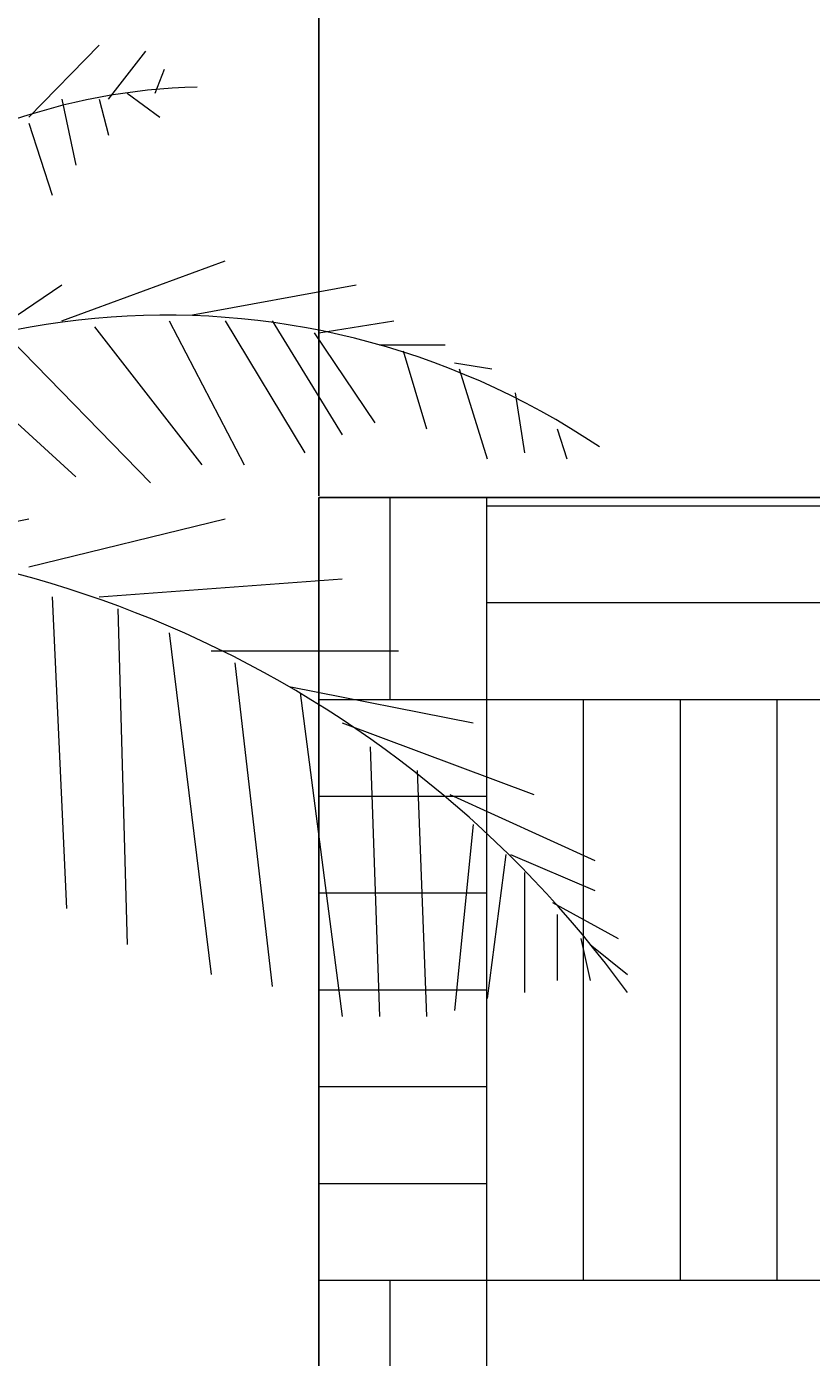
# Model space of a CAD drawing. Units: inches. Extents: x 37 to 824, y -700 to 234.
# Tile 6 of 77: x 149 to 181, y -459 to -404. Entities that reach past the tile are written whole.
import ezdxf

# ---------------------------------------------------------------- set-up
doc = ezdxf.new("R2010")
doc.units = ezdxf.units.IN
doc.header["$MEASUREMENT"] = 0
for name, color, linetype, lineweight in [('A-ANNO-DIMS', 2, 'Continuous', 18), ('A-ELEV', 3, 'Continuous', 25), ('A-ELEV-PATT', 8, 'Continuous', 13), ('A-SITE-PLNT', 3, 'Continuous', 13)]:
    doc.layers.add(name, color=color, linetype=linetype, lineweight=lineweight)
doc.styles.get("Standard").update_dxf_attribs({"font": 'arial.ttf'})
doc.dimstyles.get("Standard").update_dxf_attribs({"dimtxt": 0.18, "dimasz": 0.18, "dimexe": 0.18, "dimexo": 0.0625, "dimgap": 0.09, "dimtad": 0, "dimtih": 1, "dimtoh": 1, "dimdec": 1, "dimzin": 0, "dimdsep": 46, "dimlunit": 4, "dimtxsty": 'Standard', "dimcen": 0.09, "dimadec": 0, "dimazin": 0, "dimtfac": 1, "dimtdec": 1, "dimtofl": 0, "dimtmove": 0, "dimatfit": 3, "dimfxl": 1, "dimtolj": 1, "dimtzin": 0, "dimarcsym": 0})

# ---------------------------------------------------------------- blocks, each defined once
blk = doc.blocks.new('*U34')
for p, q in [((18.015, 195.716), (20.914, 198.689)), ((21.301, 196.459), (22.847, 198.441)), ((23.234, 196.707), (23.62, 197.698)), ((19.368, 196.459), (19.948, 193.733)), ((20.914, 196.459), (21.301, 194.972)), ((22.074, 196.707), (23.427, 195.716)), ((18.015, 195.468), (18.981, 192.494)), ((19.368, 187.29), (26.133, 189.768)), ((15.695, 186.299), (19.368, 188.777)), ((24.78, 187.538), (31.546, 188.777)), ((20.721, 187.042), (25.167, 181.343)), ((23.814, 187.29), (26.907, 181.343)), ((26.133, 187.29), (29.419, 181.838)), ((28.066, 187.29), (30.966, 182.582)), ((29.999, 186.795), (33.092, 187.29)), ((17.242, 186.547), (23.041, 180.599)), ((29.806, 186.795), (32.319, 183.078)), ((32.512, 186.299), (35.218, 186.299)), ((33.479, 186.051), (34.445, 182.83)), ((14.536, 185.803), (19.948, 180.847)), ((35.605, 185.556), (37.151, 185.308)), ((35.798, 185.308), (36.958, 181.591)), ((38.118, 184.317), (38.504, 181.838)), ((39.857, 182.83), (40.244, 181.591)), ((11.829, 177.874), (18.015, 179.113)), ((18.015, 177.13), (26.133, 179.113)), ((20.914, 175.891), (30.966, 176.635)), ((18.981, 175.891), (19.561, 163.005)), ((21.688, 175.396), (22.074, 161.518)), ((23.814, 174.404), (25.554, 160.279)), ((25.554, 173.661), (33.285, 173.661)), ((26.52, 173.165), (28.066, 159.784)), ((28.839, 172.174), (36.378, 170.687)), ((29.226, 171.926), (30.966, 158.545)), ((30.966, 170.687), (38.891, 167.713)), ((32.126, 169.696), (32.512, 158.545)), ((34.058, 168.705), (34.445, 158.545)), ((35.412, 167.713), (41.404, 164.988)), ((36.378, 166.474), (35.605, 158.792)), ((37.731, 165.235), (36.958, 159.288)), ((37.924, 165.235), (41.404, 163.749)), ((38.504, 164.492), (38.504, 159.536)), ((39.664, 163.253), (42.37, 161.766)), ((39.857, 162.757), (39.857, 160.031)), ((40.824, 161.766), (41.21, 160.031)), ((41.21, 161.518), (42.757, 160.279))]:
    blk.add_line(p, q)
for centre, radius, start, end in [((25.595, 171.567), 25.395, 91.4032, 163.882), ((23.687, 155.341), 32.188, 56.1927, 134.3213), ((5.828, 132.718), 45.639, 35.9878, 95.8227)]:
    blk.add_arc(centre, radius, start, end)
blk = doc.blocks.new('*D66')
at = {"layer": 'A-ANNO-DIMS', "color": 0, "lineweight": -2, "ltscale": 0.5, "transparency": 16777216}
for p, q in [((161.077, -423.565), (161.077, -378.38)), ((161.257, -378.56), (294.176, -378.56)), ((427.897, -378.56), (294.978, -378.56)), ((428.077, -423.565), (428.077, -378.38))]:
    blk.add_line(p, q, dxfattribs=at)
at = {"layer": 'A-ANNO-DIMS', "color": 0, "ltscale": 0.5, "transparency": 16777216}
for points in [[(161.257, -378.53), (161.257, -378.59), (161.077, -378.56)], [(427.897, -378.53), (427.897, -378.59), (428.077, -378.56)]]:
    blk.add_solid(points, dxfattribs=at)
at = {"layer": 'Defpoints', "color": 0, "ltscale": 0.5, "transparency": 16777216}
for p in [(428.077, -378.56), (161.077, -423.627), (428.077, -423.627)]:
    blk.add_point(p, dxfattribs=at)
at = {"layer": 'A-ANNO-DIMS', "color": 0, "ltscale": 0.5, "transparency": 16777216, "insert": (294.577, -378.56), "char_height": 0.18, "attachment_point": 5}
blk.add_mtext('\\A1;22\'-3"', dxfattribs=at)

msp = doc.modelspace()

# ---------------------------------------------------------------- hatches: boundary and pattern name
at = {"layer": 'A-ELEV-PATT', "ltscale": 0.5}
h = msp.add_hatch(dxfattribs=at)
h.set_pattern_fill('AR-PARQ1', color=256, scale=2)
h.paths.add_polyline_path([(428.077, -423.627), (161.077, -423.627), (161.077, -459.627), (428.077, -459.627)])

# ---------------------------------------------------------------- linework, layer by layer
at = {"layer": 'A-ELEV', "ltscale": 0.5}
msp.add_lwpolyline([(161.077, -423.627), (428.077, -423.627), (428.077, -459.627), (161.077, -459.627)], close=True, dxfattribs=at)

# ---------------------------------------------------------------- block references
at = {"layer": 'A-SITE-PLNT'}
msp.add_blockref('*U34', (131.077, -603.627), dxfattribs=at)

# ---------------------------------------------------------------- dimensions: what is measured, and where the dimension line sits
at = {"layer": 'A-ANNO-DIMS', "ltscale": 0.5}
dim = msp.add_linear_dim(base=(428.077, -378.56), p1=(161.077, -423.627), p2=(428.077, -423.627), dimstyle='Standard', override={"dimdec": 1, "dimlfac": 1, "dimrnd": 0, "dimzin": 1, "dimdsep": 46, "dimlunit": 4, "dimfrac": 2}, dxfattribs=at)
dim.commit()
dim.dimension.update_dxf_attribs({"geometry": '*D66', "text_midpoint": (294.577, -378.56)})

doc.saveas('drawing.dxf')
